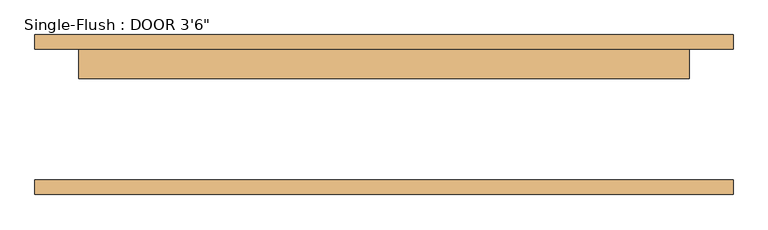
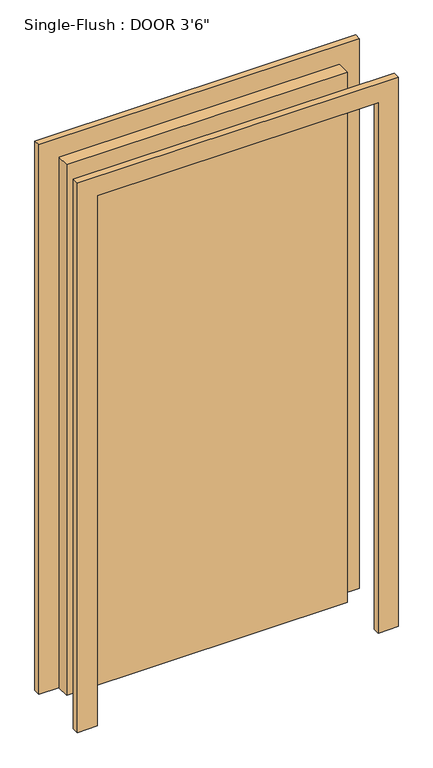
"""IFC4 building model written with IfcOpenShell, lengths in millimetres: door geometry."""

from ifc_helpers import new_model, si_unit, frame, origin, origin_with_axes, place, context, project, spatial, polyline, outline, extrude, source, transform, mapped, element, save


def door_9d399b00(model_context):
    return source(origin(), model_context, "Body", "SweptSolid", [
        extrude(outline(polyline([(2209.8, -609.6), (0.0, -609.6), (0.0, -533.4), (2133.6, -533.4), (2133.6, 533.4), (0.0, 533.4), (0.0, 609.6), (2209.8, 609.6), (2209.8, -609.6)])), frame((0.0, 114.3, 0.0), z_axis=(0.0, 1.0, 0.0), x_axis=(0.0, 0.0, 1.0)), (0.0, 0.0, 1.0), 25.4),
        extrude(outline(polyline([(2209.8, 609.6), (2209.8, -609.6), (0.0, -609.6), (0.0, -533.4), (2133.6, -533.4), (2133.6, 533.4), (0.0, 533.4), (0.0, 609.6), (2209.8, 609.6)])), frame((0.0, -139.7, 0.0), z_axis=(0.0, 1.0, 0.0), x_axis=(0.0, 0.0, 1.0)), (0.0, 0.0, 1.0), 25.4),
        extrude(outline(polyline([(533.4, 63.5), (-533.4, 63.5), (-533.4, 114.3), (533.4, 114.3), (533.4, 63.5)])), origin_with_axes(), (0.0, 0.0, 1.0), 2133.6),
    ])


if __name__ == "__main__":
    model = new_model("IFC4")
    model_context = context("Model", 3, world=origin())
    ifc_project = project(units=[si_unit("LENGTHUNIT", "METRE", prefix="MILLI")], contexts=[model_context])
    site = spatial("IfcSite", under=ifc_project)
    building = spatial("IfcBuilding", under=site)
    placement = place(None, origin())
    door_shape = door_9d399b00(model_context)
    element("IfcDoor", 1, ObjectType="Single-Flush : DOOR 3'6\"", at=placement, inside=building, context=model_context, shape_type="MappedRepresentation", body=[
        mapped(door_shape, transform((0.0, 0.0, 0.0), x_axis=(1.0, 0.0, 0.0), y_axis=(0.0, 1.0, 0.0), z_axis=(0.0, 0.0, 1.0))),
    ])
    save(model, "model.ifc")

# Revit data of these elements
# Type "Single-Flush : DOOR 3'6\""
#   Type Mark = "9"
#   Construction Type Id = "MDOOR"
#   Assembly Code = "C1020"
#   Analytic Construction = "Metal"
#   Thickness = 0' - 2"
#   Heat Transfer Coefficient (U) = 0.651978 BTU/(h·ft²·°F)
#   Height = 7' - 0"
#   Trim Projection Ext = 0' - 1"
#   Trim Projection Int = 0' - 1"
#   Trim Width = 0' - 3"
#   Width = 3' - 6"
#   Define Thermal Properties by = 1
#   Door Material = Door - Panel
#   Frame Material = Door - Frame
#   Visual Light Transmittance = 0
#   Solar Heat Gain Coefficient = 0
#   Function = (empty or 0)
#   Wall Closure = (empty or 0)
# Element 1 (IfcDoor, "Single-Flush : DOOR 3'6\"")
#   Materials on its faces: "Door - Frame", "Door - Panel"
# Materials
#   "Door - Panel": class "Wood", colour RGB 210 159 95, transparency 0, Cost = 0
#   "Door - Frame": colour RGB 118 70 51, transparency 0, Cost = 0
